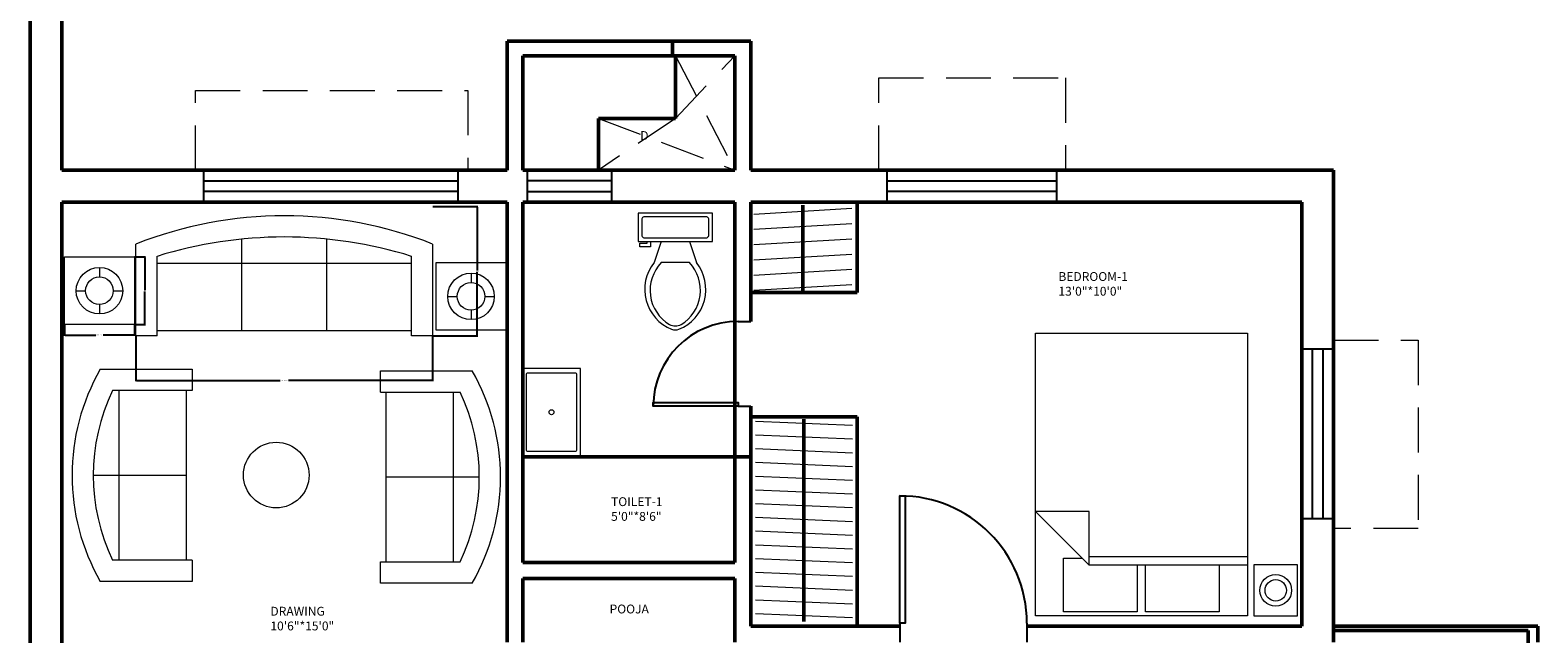
# Model space of a CAD drawing. Units: inches. Extents: x 291 to 2631, y 456 to 2623.
# Tile 13 of 22: x 2168 to 2595, y 1367 to 1538. Entities that reach past the tile are written whole.
import ezdxf

# ---------------------------------------------------------------- set-up
doc = ezdxf.new("R2010")
doc.units = ezdxf.units.IN
doc.linetypes.add('DASHED', pattern=[19.05, 12.7, -6.35])
for name, color, linetype, lineweight in [('A-ANNO-DIMS', 2, 'Continuous', 18), ('A-ANNO-TEXT', 3, 'Continuous', 25), ('A-AREA-IDEN', 7, 'Continuous', 25), ('A-DOOR', 3, 'Continuous', 25), ('A-FLOR-FIXT', 9, 'Continuous', 18), ('A-FLOR-OVHD', 1, 'DASHED', 18), ('A-FURN', 8, 'Continuous', 18), ('A-GLAZ', 4, 'Continuous', 25), ('A-WALL', 7, 'Continuous', 50)]:
    doc.layers.add(name, color=color, linetype=linetype, lineweight=lineweight)
doc.styles.get("Standard").update_dxf_attribs({"font": 'arial.ttf'})
doc.dimstyles.get("Standard").update_dxf_attribs({"dimtxt": 0.18, "dimasz": 0.18, "dimexe": 0.18, "dimexo": 0.0625, "dimgap": 0.09, "dimtad": 0, "dimtih": 1, "dimtoh": 1, "dimdec": 4, "dimzin": 0, "dimdsep": 46, "dimtxsty": 'Standard', "dimcen": 0.09, "dimadec": 0, "dimazin": 0, "dimtfac": 1, "dimtdec": 4, "dimtofl": 0, "dimtmove": 0, "dimatfit": 3, "dimfxl": 1, "dimtolj": 1, "dimtzin": 0, "dimarcsym": 0})

# ---------------------------------------------------------------- blocks, each defined once
blk = doc.blocks.new('*U2')
for p, q in [((0, 0), (0, -6)), ((40, 0), (40, -6))]:
    blk.add_line(p, q)
blk.add_lwpolyline([(0, 0), (0, 40), (1.75, 40), (1.75, 0)], close=True)
blk.add_arc((0, 0), 40, 0, 90)
blk = doc.blocks.new('Sofa - Roundback 7 ft.')
for p, q in [((-12.00002, -32.4421), (-12.00003, -6.5971)), ((11.99997, -32.4421), (11.99998, -6.5971)), ((-36.000027, -34), (-36.000027, -11.4696)), ((35.99998, -34), (35.99998, -11.4696)), ((-35.999844, -13.3819), (35.9998, -13.3819)), ((-36.000027, -32.4421), (35.99998, -32.4421))]:
    blk.add_line(p, q)
for points in [[(-36.000027, -34), (-42.000027, -34), (-42.000027, -8)], [(41.99998, -8), (41.99998, -34), (35.99998, -34)]]:
    blk.add_lwpolyline(points)
for centre, radius, start, end in [((0, -114.25), 114.25, 68.43141, 111.5686), ((-0.00001, -127.1968), 121.1968, 72.72033, 107.2797)]:
    blk.add_arc(centre, radius, start, end)
blk = doc.blocks.new('Sofa - Roundback Loveseat 5 ft.')
for p, q in [((0, -32.44198), (0, -5.99998)), ((-24, -33.99998), (-24, -11.46958)), ((24.00004, -33.99998), (24.00004, -11.46958)), ((-23.9998, -13.38178), (23.99986, -13.38178)), ((-24, -32.44198), (24.00004, -32.44198))]:
    blk.add_line(p, q)
for points in [[(-24, -33.99998), (-30, -33.99998), (-30, -7.99998)], [(30.00004, -7.99998), (30.00004, -33.99998), (24.00004, -33.99998)]]:
    blk.add_lwpolyline(points)
for centre, radius, start, end in [((0, -60.24998), 60.24998, 60.13715, 119.8628), ((0, -61.38438), 55.38444, 64.32083, 115.6792)]:
    blk.add_arc(centre, radius, start, end)
blk = doc.blocks.new('Toilet - top')
for p, q in [((9.5, -6), (9.5, -2)), ((-10, -8.5), (-8, -8.5)), ((-10, -9.5), (-10, -8.5)), ((-8, -8.5), (-8, -8)), ((-7, -8), (-7, -9.5)), ((-4, -8), (-6, -14)), ((4, -8), (6, -14)), ((-7, -9.5), (-10, -9.5)), ((4, -14), (-4, -14))]:
    blk.add_line(p, q)
blk.add_lwpolyline([(10.5, -8), (10.5, 0), (-10.5, 0), (-10.5, -8)], close=True)
for points in [[(-9.5, -2), (-9.5, -6)], [(8.5, -1), (-8.5, -1)], [(-8.5, -7), (8.5, -7)]]:
    blk.add_lwpolyline(points)
for centre, radius, start, end in [((-8.62, -1.88), 0.884, 81.8699, 188.1301), ((8.62, -1.88), 0.884, 351.8699, 98.1301), ((-8.62, -6.12), 0.884, 171.8699, 278.1301), ((8.62, -6.12), 0.884, 261.8699, 8.1301), ((3.52, -21.58), 12.17, 141.4691, 247.9714), ((4.2, -21.82), 11.33, 136.3677, 238.9468), ((-3.52, -21.58), 12.17, 292.0284, 38.5307), ((-4.2, -21.82), 11.33, 301.053, 43.6321), ((0, -27.88), 4, 245.7318, 294.2682), ((0, -29), 4, 254.8605, 285.1395)]:
    blk.add_arc(centre, radius, start, end)
blk = doc.blocks.new('Bed - Queen')
for p, q in [((0, -80.00003), (0, 0)), ((0, 0), (59.99999, 0)), ((59.99999, 0), (59.99999, -80.00003)), ((7.99999, -1.2), (28.79998, -1.2)), ((7.99999, -14.4), (7.99999, -1.2)), ((28.79998, -1.2), (28.79998, -14.4)), ((31.19999, -1.2), (51.99999, -1.2)), ((31.19999, -14.4), (31.19999, -1.2)), ((51.99999, -1.2), (51.99999, -16.4)), ((0, -14.4), (44.8, -14.4)), ((44.8, -16.8), (0, -16.8)), ((59.99999, -29.6), (44.8, -14.4)), ((44.8, -14.4), (44.8, -29.6)), ((51.99999, -16.4), (46.79936, -16.4)), ((44.8, -29.6), (59.99999, -29.6)), ((59.99999, -80.00003), (0, -80.00003))]:
    blk.add_line(p, q)
blk = doc.blocks.new('WIN-1800')
for p, q in [((0, 9), (72, 9)), ((0, 0), (0, 9)), ((72, 9), (72, 0)), ((0, 6), (72, 6)), ((72, 3), (0, 3)), ((72, 0), (0, 0))]:
    blk.add_line(p, q)
blk = doc.blocks.new('WIN-1200')
for p, q in [((0, 0), (0, 48)), ((0, 48), (9, 48)), ((3, 0), (3, 48)), ((6, 48), (6, 0)), ((9, 48), (9, 0)), ((9, 0), (0, 0))]:
    blk.add_line(p, q)
blk = doc.blocks.new('WIN-600')
for p, q in [((24, 9), (0, 9)), ((0, 9), (0, 0)), ((24, 0), (24, 9)), ((24, 6), (0, 6)), ((0, 3), (24, 3)), ((0, 0), (24, 0))]:
    blk.add_line(p, q)
blk = doc.blocks.new('LAMP-C')
for p, q in [((9.9, 16.15), (9.9, 13.47)), ((3.32, 9.57), (5.99, 9.57)), ((13.8, 9.57), (16.48, 9.57)), ((9.9, 5.66), (9.9, 2.99))]:
    blk.add_line(p, q)
blk.add_lwpolyline([(0, 19.13), (19.79, 19.13), (19.79, 0), (0, 0)], close=True)
for radius in [6.58, 3.91]:
    blk.add_circle((9.9, 9.57), radius)
blk = doc.blocks.new('*D34')
at = {"layer": 'A-ANNO-DIMS', "color": 0, "lineweight": -2, "transparency": 16777216}
for p, q in [((2198.16, 1451.07), (2198.16, 1438.36)), ((2282.16, 1451.07), (2282.16, 1438.36)), ((2198.34, 1438.54), (2238.96, 1438.54)), ((2281.98, 1438.54), (2241.35, 1438.54))]:
    blk.add_line(p, q, dxfattribs=at)
at = {"layer": 'A-ANNO-DIMS', "color": 0, "transparency": 16777216}
for points in [[(2198.34, 1438.57), (2198.34, 1438.51), (2198.16, 1438.54)], [(2281.98, 1438.57), (2281.98, 1438.51), (2282.16, 1438.54)]]:
    blk.add_solid(points, dxfattribs=at)
at = {"layer": 'DEFPOINTS', "color": 0, "transparency": 16777216}
for p in [(2198.16, 1451.14), (2282.16, 1451.14), (2282.16, 1438.54)]:
    blk.add_point(p, dxfattribs=at)
at = {"layer": 'A-ANNO-DIMS', "color": 0, "transparency": 16777216, "insert": (2240.16, 1438.54), "char_height": 0.18, "attachment_point": 5}
blk.add_mtext('\\A1;SOFA 7 FT 84 TYP.', dxfattribs=at)
blk = doc.blocks.new('*D35')
at = {"layer": 'A-ANNO-DIMS', "color": 0, "lineweight": -2, "transparency": 16777216}
for p, q in [((2282.22, 1487.8), (2294.94, 1487.8)), ((2294.76, 1487.62), (2294.76, 1469.65)), ((2294.76, 1451.32), (2294.76, 1469.29)), ((2282.22, 1451.14), (2294.94, 1451.14))]:
    blk.add_line(p, q, dxfattribs=at)
at = {"layer": 'A-ANNO-DIMS', "color": 0, "transparency": 16777216}
for points in [[(2294.73, 1487.62), (2294.79, 1487.62), (2294.76, 1487.8)], [(2294.73, 1451.32), (2294.79, 1451.32), (2294.76, 1451.14)]]:
    blk.add_solid(points, dxfattribs=at)
at = {"layer": 'DEFPOINTS', "color": 0, "transparency": 16777216}
for p in [(2282.16, 1487.8), (2294.76, 1487.8), (2282.16, 1451.14)]:
    blk.add_point(p, dxfattribs=at)
at = {"layer": 'A-ANNO-DIMS', "color": 0, "transparency": 16777216, "insert": (2294.76, 1469.47), "char_height": 0.18, "attachment_point": 5}
blk.add_mtext('\\A1;37 TYP.', dxfattribs=at)
blk = doc.blocks.new('*D48')
at = {"layer": 'A-ANNO-DIMS', "color": 0, "lineweight": -2, "transparency": 16777216}
for p, q in [((2177.92, 1454.31), (2177.92, 1451.22)), ((2178.1, 1451.4), (2186.79, 1451.4)), ((2197.53, 1451.4), (2188.84, 1451.4)), ((2197.71, 1454.31), (2197.71, 1451.22))]:
    blk.add_line(p, q, dxfattribs=at)
at = {"layer": 'A-ANNO-DIMS', "color": 0, "transparency": 16777216}
for points in [[(2178.1, 1451.43), (2178.1, 1451.37), (2177.92, 1451.4)], [(2197.53, 1451.43), (2197.53, 1451.37), (2197.71, 1451.4)]]:
    blk.add_solid(points, dxfattribs=at)
at = {"layer": 'DEFPOINTS', "color": 0, "transparency": 16777216}
for p in [(2177.92, 1454.37), (2197.71, 1454.37), (2197.71, 1451.4)]:
    blk.add_point(p, dxfattribs=at)
at = {"layer": 'A-ANNO-DIMS', "color": 0, "transparency": 16777216, "insert": (2187.81, 1451.4), "char_height": 0.18, "attachment_point": 5}
blk.add_mtext('\\A1;LAMP C 20 TYP.', dxfattribs=at)
blk = doc.blocks.new('*D49')
at = {"layer": 'A-ANNO-DIMS', "color": 0, "lineweight": -2, "transparency": 16777216}
for p, q in [((2197.77, 1473.51), (2200.86, 1473.51)), ((2200.68, 1473.33), (2200.68, 1464.12)), ((2200.68, 1454.55), (2200.68, 1463.76)), ((2197.77, 1454.37), (2200.86, 1454.37))]:
    blk.add_line(p, q, dxfattribs=at)
at = {"layer": 'A-ANNO-DIMS', "color": 0, "transparency": 16777216}
for points in [[(2200.65, 1473.33), (2200.71, 1473.33), (2200.68, 1473.51)], [(2200.65, 1454.55), (2200.71, 1454.55), (2200.68, 1454.37)]]:
    blk.add_solid(points, dxfattribs=at)
at = {"layer": 'DEFPOINTS', "color": 0, "transparency": 16777216}
for p in [(2197.71, 1473.51), (2200.68, 1473.51), (2197.71, 1454.37)]:
    blk.add_point(p, dxfattribs=at)
at = {"layer": 'A-ANNO-DIMS', "color": 0, "transparency": 16777216, "insert": (2200.68, 1463.94), "char_height": 0.18, "attachment_point": 5}
blk.add_mtext('\\A1;19 TYP.', dxfattribs=at)

msp = doc.modelspace()

# ---------------------------------------------------------------- linework, layer by layer
at = {"layer": 'A-FLOR-OVHD'}
for p, q in [((2350.88, 1530.4), (2367.71, 1498.02)), ((2350.88, 1512.7), (2367.71, 1530.4)), ((2408.44, 1498.02), (2408.44, 1524.15)), ((2408.44, 1524.15), (2461.33, 1524.15)), ((2461.33, 1524.15), (2461.33, 1498.02)), ((2214.99, 1498.02), (2214.99, 1520.61)), ((2214.99, 1520.61), (2292.1, 1520.61)), ((2292.1, 1520.61), (2292.1, 1498.02)), ((2350.88, 1512.7), (2329.07, 1498.02)), ((2329.07, 1512.7), (2367.71, 1498.02)), ((2537.21, 1449.96), (2561.18, 1449.96)), ((2561.18, 1449.96), (2561.18, 1396.64)), ((2561.18, 1396.64), (2537.21, 1396.64))]:
    msp.add_line(p, q, dxfattribs=at)
at = {"layer": 'A-FURN'}
for p, q in [((2373.11, 1485.62), (2400.85, 1487.25)), ((2373.11, 1481.31), (2400.85, 1482.94)), ((2373.11, 1477), (2400.85, 1478.63)), ((2373.11, 1472.69), (2400.85, 1474.32)), ((2373.11, 1468.38), (2400.85, 1470.01)), ((2373.11, 1464.07), (2400.85, 1465.7)), ((2373.56, 1427.06), (2400.98, 1425.9)), ((2373.56, 1423.18), (2400.98, 1422.01)), ((2373.56, 1419.29), (2400.98, 1418.12)), ((2373.56, 1415.4), (2400.98, 1414.24)), ((2373.56, 1411.52), (2400.98, 1410.35)), ((2373.56, 1407.63), (2400.98, 1406.47)), ((2373.56, 1403.75), (2400.98, 1402.58)), ((2373.56, 1399.86), (2400.98, 1398.7)), ((2373.56, 1395.98), (2400.98, 1394.81)), ((2373.56, 1392.09), (2400.98, 1390.93)), ((2373.56, 1388.21), (2400.98, 1387.04)), ((2373.56, 1384.32), (2400.98, 1383.16)), ((2373.56, 1380.44), (2400.98, 1379.27)), ((2373.56, 1376.55), (2400.98, 1375.39)), ((2373.56, 1372.67), (2400.98, 1371.5))]:
    msp.add_line(p, q, dxfattribs=at)
for points in [[(2307.71, 1416.97), (2324.04, 1416.97), (2324.04, 1441.9), (2307.71, 1441.9)], [(2514.67, 1371.93), (2527.04, 1371.93), (2527.04, 1386.42), (2514.67, 1386.42)]]:
    msp.add_lwpolyline(points, close=True, dxfattribs=at)
msp.add_lwpolyline([(2309.21, 1440.73), (2322.39, 1440.73, -0.414214), (2322.89, 1440.23), (2322.89, 1418.93, -0.414214), (2322.39, 1418.43), (2309.21, 1418.43, -0.414214), (2308.71, 1418.93), (2308.71, 1440.23, -0.414214)], format="xyb", close=True, dxfattribs=at)
for centre, radius in [((2315.8, 1429.58), 0.7), ((2237.88, 1411.79), 9.28), ((2520.85, 1379.18), 4.49), ((2520.85, 1379.18), 3.03)]:
    msp.add_circle(centre, radius, dxfattribs=at)
at = {"layer": 'A-WALL'}
for p, q in [((2177.21, 1659.64), (2177.21, 1498.02)), ((2168.21, 1650.64), (2168.21, 1112.52)), ((2303.21, 1498.02), (2303.21, 1534.55)), ((2303.21, 1534.55), (2372.21, 1534.55)), ((2350.09, 1534.55), (2350.09, 1530.4)), ((2372.21, 1534.55), (2372.21, 1498.02)), ((2307.71, 1498.02), (2307.71, 1530.4)), ((2307.71, 1530.4), (2367.71, 1530.4)), ((2350.88, 1530.4), (2350.88, 1512.7)), ((2367.71, 1530.4), (2367.71, 1498.02)), ((2350.88, 1512.7), (2329.07, 1512.7)), ((2329.07, 1512.7), (2329.07, 1498.02)), ((2177.21, 1498.02), (2303.21, 1498.02)), ((2307.71, 1498.02), (2367.71, 1498.02)), ((2372.21, 1498.02), (2537.21, 1498.02)), ((2537.21, 1498.02), (2537.21, 1364.52)), ((2177.21, 1489.02), (2303.21, 1489.02)), ((2177.21, 1489.02), (2177.21, 1309.02)), ((2303.21, 1489.02), (2303.21, 1364.52)), ((2307.71, 1489.02), (2307.71, 1387.02)), ((2307.71, 1489.02), (2367.71, 1489.02)), ((2367.71, 1489.02), (2367.71, 1387.02)), ((2372.21, 1489.02), (2372.21, 1455.27)), ((2372.21, 1489.02), (2372.21, 1455.27)), ((2372.21, 1489.02), (2528.21, 1489.02)), ((2386.98, 1488.13), (2386.98, 1463.93)), ((2402.31, 1463.4), (2402.31, 1489.02)), ((2528.21, 1489.02), (2528.21, 1369.02)), ((2372.21, 1463.4), (2402.31, 1463.4)), ((2372.21, 1431.27), (2372.21, 1369.02)), ((2372.21, 1431.27), (2372.21, 1369.02)), ((2372.21, 1428.3), (2402.31, 1428.3)), ((2387.27, 1427.59), (2387.27, 1370.34)), ((2402.31, 1428.3), (2402.31, 1369.02)), ((2307.71, 1416.97), (2372.21, 1416.97)), ((2307.71, 1387.02), (2367.71, 1387.02)), ((2307.71, 1382.52), (2367.71, 1382.52)), ((2307.71, 1382.52), (2307.71, 1364.52)), ((2367.71, 1382.52), (2367.71, 1364.52)), ((2372.21, 1369.02), (2414.38, 1369.02)), ((2450.38, 1369.02), (2528.21, 1369.02)), ((2537.21, 1369.02), (2595.05, 1369.02)), ((2537.21, 1367.87), (2592.31, 1367.87)), ((2592.31, 1367.87), (2592.31, 1248.02)), ((2595.05, 1369.02), (2595.05, 1364.52))]:
    msp.add_line(p, q, dxfattribs=at)

# ---------------------------------------------------------------- block references
at = {"layer": 'A-DOOR', "xscale": 0.6, "yscale": 0.6, "zscale": 0.6, "rotation": 90.00000000000003}
msp.add_blockref('*U2', (2368.61, 1431.27), dxfattribs=at)
at = {"layer": 'A-DOOR', "xscale": 0.9, "yscale": 0.9, "zscale": 0.9}
msp.add_blockref('*U2', (2414.38, 1369.92), dxfattribs=at)
at = {"layer": 'A-FLOR-FIXT'}
msp.add_blockref('Toilet - top', (2350.85, 1485.89), dxfattribs=at)
at = {"layer": 'A-FURN'}
for name, p in [('Sofa - Roundback 7 ft.', (2240.16, 1485.14)), ('LAMP-C', (2177.92, 1454.37)), ('LAMP-C', (2283.13, 1452.77))]:
    msp.add_blockref(name, p, dxfattribs=at)
for name, p, rotation in [('Bed - Queen', (2512.8, 1371.93), 180), ('Sofa - Roundback Loveseat 5 ft.', (2180.06, 1411.72), 90), ('Sofa - Roundback Loveseat 5 ft.', (2301.37, 1411.25), 270.0000000000006)]:
    msp.add_blockref(name, p, dxfattribs=dict(at, rotation=rotation))
at = {"layer": 'A-GLAZ'}
msp.add_blockref('WIN-1800', (2217.33, 1489.02), dxfattribs=at)
for name, p, rotation in [('WIN-600', (2332.9, 1498.02), 180), ('WIN-1200', (2410.79, 1498.02), 270), ('WIN-1200', (2537.21, 1447.46), 180)]:
    msp.add_blockref(name, p, dxfattribs=dict(at, rotation=rotation))

# ---------------------------------------------------------------- texts
at = {"layer": 'A-ANNO-TEXT', "insert": (2340.92, 1509.09), "char_height": 2.5, "attachment_point": 1}
msp.add_mtext_dynamic_manual_height_columns('D', width=2.2039, gutter_width=12.5, heights=[0], dxfattribs=at)
at = {"layer": 'A-AREA-IDEN', "char_height": 2.5, "attachment_point": 1}
for s, width, insert in [('BEDROOM-1\\P13\'0"*10\'0"', 63.0881, (2459.31, 1469.21)), ('TOILET-1\\P5\'0"*8\'6"', 44.7582, (2332.67, 1405.52)), ('DRAWING\\P10\'6"*15\'0"', 59.4768, (2236.22, 1374.53)), ('POOJA', 32.2378, (2332.25, 1375.16))]:
    msp.add_mtext_dynamic_manual_height_columns(s, width=width, gutter_width=12.5, heights=[0], dxfattribs=dict(at, insert=insert))

# ---------------------------------------------------------------- dimensions: what is measured, and where the dimension line sits
at = {"layer": 'A-ANNO-DIMS'}
for base, p1, p2, picture, middle in [((2294.76, 1487.8), (2282.16, 1451.14), (2282.16, 1487.8), '*D35', (2294.76, 1469.47)), ((2200.68, 1473.51), (2197.71, 1454.37), (2197.71, 1473.51), '*D49', (2200.68, 1463.94))]:
    dim = msp.add_linear_dim(base=base, p1=p1, p2=p2, angle=90, text='<> TYP.', dimstyle='Standard', override={"dimdec": 0, "dimlfac": 1, "dimrnd": 0, "dimzin": 0, "dimdsep": 46, "dimlunit": 2}, dxfattribs=at)
    dim.commit()
    dim.dimension.update_dxf_attribs({"geometry": picture, "text_midpoint": middle})
for base, p1, p2, text, picture, middle in [((2197.71, 1451.4), (2177.92, 1454.37), (2197.71, 1454.37), 'LAMP C <> TYP.', '*D48', (2187.81, 1451.4)), ((2282.16, 1438.54), (2198.16, 1451.14), (2282.16, 1451.14), 'SOFA 7 FT <> TYP.', '*D34', (2240.16, 1438.54))]:
    dim = msp.add_linear_dim(base=base, p1=p1, p2=p2, text=text, dimstyle='Standard', override={"dimdec": 0, "dimlfac": 1, "dimrnd": 0, "dimzin": 0, "dimdsep": 46, "dimlunit": 2}, dxfattribs=at)
    dim.commit()
    dim.dimension.update_dxf_attribs({"geometry": picture, "text_midpoint": middle})

doc.saveas('drawing.dxf')
